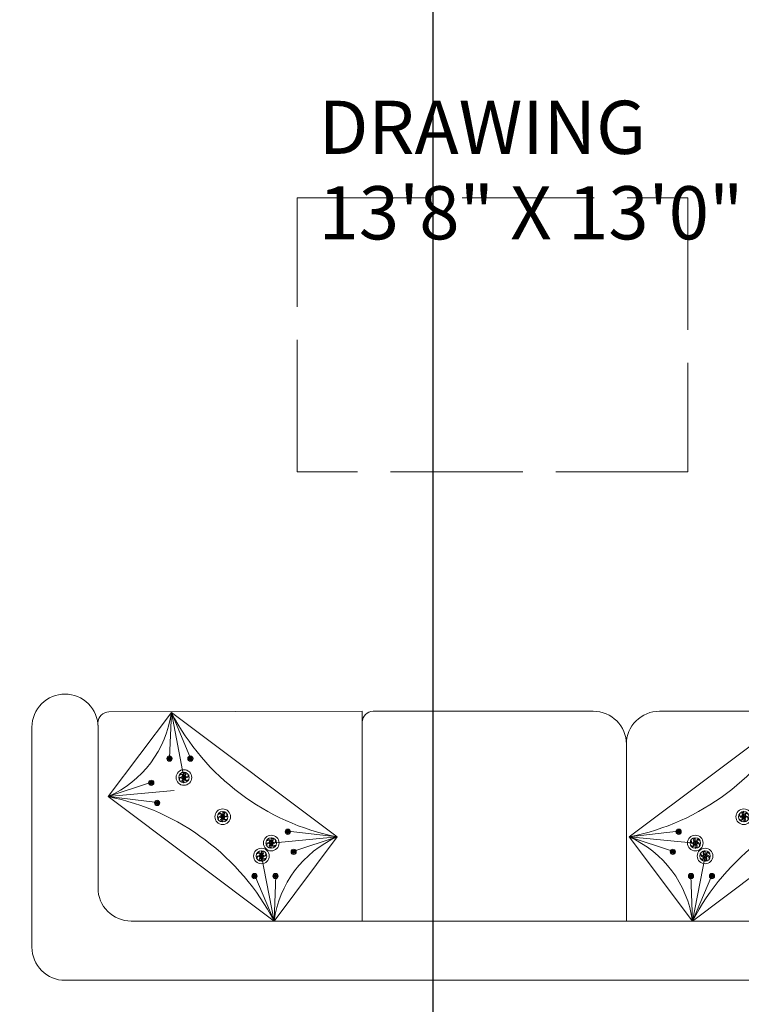
# Model space of a CAD drawing. Units: inches. Extents: x -61 to 1599, y -1316 to 257.
# Tile 132 of 204: x 418 to 484, y -166 to -77. Entities that reach past the tile are written whole.
import ezdxf

# ---------------------------------------------------------------- set-up
doc = ezdxf.new("R2010")
doc.units = ezdxf.units.IN
doc.header["$MEASUREMENT"] = 0
doc.linetypes.add('ACAD_ISO02W100', pattern=[15, 12, -3])
for name, color, linetype, lineweight in [('A-ANNO-DIMS', 2, 'Continuous', 18), ('A-AREA-IDEN', 1, 'Continuous', 18), ('A-FURN-LOW', 83, 'ACAD_ISO02W100', 18), ('FURNITURE', 83, 'Continuous', 18)]:
    doc.layers.add(name, color=color, linetype=linetype, lineweight=lineweight)
doc.layers.add('FUR', color=83, linetype='Continuous')
doc.styles.get("Standard").update_dxf_attribs({"font": 'arial.ttf'})
doc.dimstyles.get("Standard").update_dxf_attribs({"dimtxt": 0.18, "dimasz": 0.18, "dimexe": 0.18, "dimexo": 0.0625, "dimgap": 0.09, "dimtad": 0, "dimtih": 1, "dimtoh": 1, "dimdec": 0, "dimzin": 0, "dimdsep": 46, "dimlunit": 3, "dimtxsty": 'Standard', "dimcen": 0.09, "dimadec": 0, "dimazin": 0, "dimtfac": 1, "dimtdec": 0, "dimtofl": 0, "dimtmove": 0, "dimatfit": 3, "dimfxl": 1, "dimtolj": 1, "dimtzin": 0, "dimarcsym": 0})

# ---------------------------------------------------------------- blocks, each defined once
blk = doc.blocks.new('*U152')
at = {"layer": 'FUR'}
blk.add_open_spline([(0.005, 0.08), (-0.03, 0.048), (-0.098, -0.015), (0.075, -0.018), (0.024, -0.063), (0.005, -0.08)], degree=3, knots=[0, 0, 0, 0, 0.0954578, 0.1898773, 0.2470677, 0.2470677, 0.2470677, 0.2470677], dxfattribs=at)
blk = doc.blocks.new('*U153')
at = {"layer": 'FUR', "transparency": 16777216}
for p, rotation in [((222.173, -79.977), 60), ((222.178, -80.056), 120), ((222.25, -80.092), 180), ((222.312, -79.968), 300), ((222.317, -80.048), 240)]:
    blk.add_blockref('*U152', p, dxfattribs=dict(at, rotation=rotation))
blk.add_blockref('*U152', (222.24, -79.932), dxfattribs=at)
blk = doc.blocks.new('*U154')
at = {"layer": 'FUR'}
blk.add_open_spline([(0.005, 0.08), (-0.03, 0.048), (-0.098, -0.015), (0.075, -0.018), (0.024, -0.063), (0.005, -0.08)], degree=3, knots=[0, 0, 0, 0, 0.0954578, 0.1898773, 0.2470677, 0.2470677, 0.2470677, 0.2470677], dxfattribs=at)
blk = doc.blocks.new('*U155')
at = {"layer": 'FUR', "transparency": 16777216}
for p, rotation in [((222.173, -79.977), 60), ((222.178, -80.056), 120), ((222.25, -80.092), 180), ((222.312, -79.968), 300), ((222.317, -80.048), 240)]:
    blk.add_blockref('*U154', p, dxfattribs=dict(at, rotation=rotation))
blk.add_blockref('*U154', (222.24, -79.932), dxfattribs=at)
blk = doc.blocks.new('*U148')
at = {"layer": 'FUR'}
blk.add_open_spline([(0.005, 0.08), (-0.03, 0.048), (-0.098, -0.015), (0.075, -0.018), (0.024, -0.063), (0.005, -0.08)], degree=3, knots=[0, 0, 0, 0, 0.0954578, 0.1898773, 0.2470677, 0.2470677, 0.2470677, 0.2470677], dxfattribs=at)
blk = doc.blocks.new('*U149')
at = {"layer": 'FUR', "transparency": 16777216}
for p, rotation in [((222.173, -79.977), 60), ((222.178, -80.056), 120), ((222.25, -80.092), 180), ((222.312, -79.968), 300), ((222.317, -80.048), 240)]:
    blk.add_blockref('*U148', p, dxfattribs=dict(at, rotation=rotation))
blk.add_blockref('*U148', (222.24, -79.932), dxfattribs=at)
blk = doc.blocks.new('*U128')
at = {"layer": 'FUR'}
blk.add_open_spline([(0.015, 0.238), (-0.088, 0.143), (-0.292, -0.045), (0.224, -0.053), (0.072, -0.187), (0.015, -0.238)], degree=3, knots=[0, 0, 0, 0, 0.2846533, 0.5662105, 0.736751, 0.736751, 0.736751, 0.736751], dxfattribs=at)
blk = doc.blocks.new('*U129')
at = {"layer": 'FUR', "transparency": 16777216}
for p, rotation in [((662.517, -238.489), 60), ((662.531, -238.727), 120), ((662.745, -238.833), 180), ((662.929, -238.463), 300), ((662.944, -238.702), 240)]:
    blk.add_blockref('*U128', p, dxfattribs=dict(at, rotation=rotation))
blk.add_blockref('*U128', (662.716, -238.357), dxfattribs=at)
blk = doc.blocks.new('*U150')
at = {"layer": 'FUR'}
blk.add_open_spline([(0.005, 0.08), (-0.03, 0.048), (-0.098, -0.015), (0.075, -0.018), (0.024, -0.063), (0.005, -0.08)], degree=3, knots=[0, 0, 0, 0, 0.0954578, 0.1898773, 0.2470677, 0.2470677, 0.2470677, 0.2470677], dxfattribs=at)
blk = doc.blocks.new('*U151')
at = {"layer": 'FUR', "transparency": 16777216}
for p, rotation in [((222.173, -79.977), 60), ((222.178, -80.056), 120), ((222.25, -80.092), 180), ((222.312, -79.968), 300), ((222.317, -80.048), 240)]:
    blk.add_blockref('*U150', p, dxfattribs=dict(at, rotation=rotation))
blk.add_blockref('*U150', (222.24, -79.932), dxfattribs=at)
blk = doc.blocks.new('*U132')
at = {"layer": 'FUR'}
blk.add_open_spline([(0.015, 0.238), (-0.088, 0.143), (-0.292, -0.045), (0.224, -0.053), (0.072, -0.187), (0.015, -0.238)], degree=3, knots=[0, 0, 0, 0, 0.2846533, 0.5662105, 0.736751, 0.736751, 0.736751, 0.736751], dxfattribs=at)
blk = doc.blocks.new('*U133')
at = {"layer": 'FUR', "transparency": 16777216}
for p, rotation in [((662.517, -238.489), 60), ((662.531, -238.727), 120), ((662.745, -238.833), 180), ((662.929, -238.463), 300), ((662.944, -238.702), 240)]:
    blk.add_blockref('*U132', p, dxfattribs=dict(at, rotation=rotation))
blk.add_blockref('*U132', (662.716, -238.357), dxfattribs=at)
blk = doc.blocks.new('*U124')
at = {"layer": 'FUR'}
blk.add_open_spline([(0.005, 0.08), (-0.03, 0.048), (-0.098, -0.015), (0.075, -0.018), (0.024, -0.063), (0.005, -0.08)], degree=3, knots=[0, 0, 0, 0, 0.0954578, 0.1898773, 0.2470677, 0.2470677, 0.2470677, 0.2470677], dxfattribs=at)
blk = doc.blocks.new('*U125')
at = {"layer": 'FUR', "transparency": 16777216}
for p, rotation in [((222.173, -79.977), 60), ((222.178, -80.056), 120), ((222.25, -80.092), 180), ((222.312, -79.968), 300), ((222.317, -80.048), 240)]:
    blk.add_blockref('*U124', p, dxfattribs=dict(at, rotation=rotation))
blk.add_blockref('*U124', (222.24, -79.932), dxfattribs=at)
blk = doc.blocks.new('*U134')
at = {"layer": 'FUR'}
blk.add_open_spline([(0.015, 0.238), (-0.088, 0.143), (-0.292, -0.045), (0.224, -0.053), (0.072, -0.187), (0.015, -0.238)], degree=3, knots=[0, 0, 0, 0, 0.2846533, 0.5662105, 0.736751, 0.736751, 0.736751, 0.736751], dxfattribs=at)
blk = doc.blocks.new('*U123')
at = {"layer": 'FUR', "transparency": 16777216}
for p, rotation in [((662.517, -238.489), 60), ((662.531, -238.727), 120), ((662.745, -238.833), 180), ((662.929, -238.463), 300), ((662.944, -238.702), 240)]:
    blk.add_blockref('*U134', p, dxfattribs=dict(at, rotation=rotation))
blk.add_blockref('*U134', (662.716, -238.357), dxfattribs=at)
blk = doc.blocks.new('*U130')
at = {"layer": 'FUR'}
blk.add_open_spline([(0.015, 0.238), (-0.088, 0.143), (-0.292, -0.045), (0.224, -0.053), (0.072, -0.187), (0.015, -0.238)], degree=3, knots=[0, 0, 0, 0, 0.2846533, 0.5662105, 0.736751, 0.736751, 0.736751, 0.736751], dxfattribs=at)
blk = doc.blocks.new('*U131')
at = {"layer": 'FUR', "transparency": 16777216}
for p, rotation in [((662.517, -238.489), 60), ((662.531, -238.727), 120), ((662.745, -238.833), 180), ((662.929, -238.463), 300), ((662.944, -238.702), 240)]:
    blk.add_blockref('*U130', p, dxfattribs=dict(at, rotation=rotation))
blk.add_blockref('*U130', (662.716, -238.357), dxfattribs=at)
blk = doc.blocks.new('*U126')
at = {"layer": 'FUR'}
blk.add_open_spline([(0.005, 0.08), (-0.03, 0.048), (-0.098, -0.015), (0.075, -0.018), (0.024, -0.063), (0.005, -0.08)], degree=3, knots=[0, 0, 0, 0, 0.0954578, 0.1898773, 0.2470677, 0.2470677, 0.2470677, 0.2470677], dxfattribs=at)
blk = doc.blocks.new('*U127')
at = {"layer": 'FUR', "transparency": 16777216}
for p, rotation in [((222.173, -79.977), 60), ((222.178, -80.056), 120), ((222.25, -80.092), 180), ((222.312, -79.968), 300), ((222.317, -80.048), 240)]:
    blk.add_blockref('*U126', p, dxfattribs=dict(at, rotation=rotation))
blk.add_blockref('*U126', (222.24, -79.932), dxfattribs=at)
blk = doc.blocks.new('*U146')
at = {"layer": 'FUR'}
blk.add_open_spline([(0.005, 0.08), (-0.03, 0.048), (-0.098, -0.015), (0.075, -0.018), (0.024, -0.063), (0.005, -0.08)], degree=3, knots=[0, 0, 0, 0, 0.0954578, 0.1898773, 0.2470677, 0.2470677, 0.2470677, 0.2470677], dxfattribs=at)
blk = doc.blocks.new('*U147')
at = {"layer": 'FUR', "transparency": 16777216}
for p, rotation in [((222.173, -79.977), 60), ((222.178, -80.056), 120), ((222.25, -80.092), 180), ((222.312, -79.968), 300), ((222.317, -80.048), 240)]:
    blk.add_blockref('*U146', p, dxfattribs=dict(at, rotation=rotation))
blk.add_blockref('*U146', (222.24, -79.932), dxfattribs=at)
blk = doc.blocks.new('*U144')
at = {"layer": 'FUR'}
blk.add_open_spline([(0.005, 0.08), (-0.03, 0.048), (-0.098, -0.015), (0.075, -0.018), (0.024, -0.063), (0.005, -0.08)], degree=3, knots=[0, 0, 0, 0, 0.0954578, 0.1898773, 0.2470677, 0.2470677, 0.2470677, 0.2470677], dxfattribs=at)
blk = doc.blocks.new('*U145')
at = {"layer": 'FUR', "transparency": 16777216}
for p, rotation in [((222.173, -79.977), 60), ((222.178, -80.056), 120), ((222.25, -80.092), 180), ((222.312, -79.968), 300), ((222.317, -80.048), 240)]:
    blk.add_blockref('*U144', p, dxfattribs=dict(at, rotation=rotation))
blk.add_blockref('*U144', (222.24, -79.932), dxfattribs=at)
blk = doc.blocks.new('*U114')
at = {"layer": 'FUR'}
blk.add_open_spline([(0.005, 0.08), (-0.03, 0.048), (-0.098, -0.015), (0.075, -0.018), (0.024, -0.063), (0.005, -0.08)], degree=3, knots=[0, 0, 0, 0, 0.0954578, 0.1898773, 0.2470677, 0.2470677, 0.2470677, 0.2470677], dxfattribs=at)
blk = doc.blocks.new('*U115')
at = {"layer": 'FUR', "transparency": 16777216}
for p, rotation in [((222.173, -79.977), 60), ((222.178, -80.056), 120), ((222.25, -80.092), 180), ((222.312, -79.968), 300), ((222.317, -80.048), 240)]:
    blk.add_blockref('*U114', p, dxfattribs=dict(at, rotation=rotation))
blk.add_blockref('*U114', (222.24, -79.932), dxfattribs=at)
blk = doc.blocks.new('*U116')
at = {"layer": 'FUR'}
blk.add_open_spline([(0.005, 0.08), (-0.03, 0.048), (-0.098, -0.015), (0.075, -0.018), (0.024, -0.063), (0.005, -0.08)], degree=3, knots=[0, 0, 0, 0, 0.0954578, 0.1898773, 0.2470677, 0.2470677, 0.2470677, 0.2470677], dxfattribs=at)
blk = doc.blocks.new('*U117')
at = {"layer": 'FUR', "transparency": 16777216}
for p, rotation in [((222.173, -79.977), 60), ((222.178, -80.056), 120), ((222.25, -80.092), 180), ((222.312, -79.968), 300), ((222.317, -80.048), 240)]:
    blk.add_blockref('*U116', p, dxfattribs=dict(at, rotation=rotation))
blk.add_blockref('*U116', (222.24, -79.932), dxfattribs=at)
blk = doc.blocks.new('*U112')
at = {"layer": 'FUR'}
blk.add_open_spline([(0.005, 0.08), (-0.03, 0.048), (-0.098, -0.015), (0.075, -0.018), (0.024, -0.063), (0.005, -0.08)], degree=3, knots=[0, 0, 0, 0, 0.0954578, 0.1898773, 0.2470677, 0.2470677, 0.2470677, 0.2470677], dxfattribs=at)
blk = doc.blocks.new('*U113')
at = {"layer": 'FUR', "transparency": 16777216}
for p, rotation in [((222.173, -79.977), 60), ((222.178, -80.056), 120), ((222.25, -80.092), 180), ((222.312, -79.968), 300), ((222.317, -80.048), 240)]:
    blk.add_blockref('*U112', p, dxfattribs=dict(at, rotation=rotation))
blk.add_blockref('*U112', (222.24, -79.932), dxfattribs=at)
blk = doc.blocks.new('*U142')
at = {"layer": 'FUR'}
blk.add_open_spline([(0.015, 0.238), (-0.088, 0.143), (-0.292, -0.045), (0.224, -0.053), (0.072, -0.187), (0.015, -0.238)], degree=3, knots=[0, 0, 0, 0, 0.2846533, 0.5662105, 0.736751, 0.736751, 0.736751, 0.736751], dxfattribs=at)
blk = doc.blocks.new('*U143')
at = {"layer": 'FUR', "transparency": 16777216}
for p, rotation in [((662.517, -238.489), 60), ((662.531, -238.727), 120), ((662.745, -238.833), 180), ((662.929, -238.463), 300), ((662.944, -238.702), 240)]:
    blk.add_blockref('*U142', p, dxfattribs=dict(at, rotation=rotation))
blk.add_blockref('*U142', (662.716, -238.357), dxfattribs=at)
blk = doc.blocks.new('*U158')
at = {"layer": 'FUR'}
blk.add_open_spline([(0.015, 0.238), (-0.088, 0.143), (-0.292, -0.045), (0.224, -0.053), (0.072, -0.187), (0.015, -0.238)], degree=3, knots=[0, 0, 0, 0, 0.2846533, 0.5662105, 0.736751, 0.736751, 0.736751, 0.736751], dxfattribs=at)
blk = doc.blocks.new('*U109')
at = {"layer": 'FUR', "transparency": 16777216}
for p, rotation in [((662.517, -238.489), 60), ((662.531, -238.727), 120), ((662.745, -238.833), 180), ((662.929, -238.463), 300), ((662.944, -238.702), 240)]:
    blk.add_blockref('*U158', p, dxfattribs=dict(at, rotation=rotation))
blk.add_blockref('*U158', (662.716, -238.357), dxfattribs=at)
blk = doc.blocks.new('*U110')
at = {"layer": 'FUR'}
blk.add_open_spline([(0.005, 0.08), (-0.03, 0.048), (-0.098, -0.015), (0.075, -0.018), (0.024, -0.063), (0.005, -0.08)], degree=3, knots=[0, 0, 0, 0, 0.0954578, 0.1898773, 0.2470677, 0.2470677, 0.2470677, 0.2470677], dxfattribs=at)
blk = doc.blocks.new('*U111')
at = {"layer": 'FUR', "transparency": 16777216}
for p, rotation in [((222.173, -79.977), 60), ((222.178, -80.056), 120), ((222.25, -80.092), 180), ((222.312, -79.968), 300), ((222.317, -80.048), 240)]:
    blk.add_blockref('*U110', p, dxfattribs=dict(at, rotation=rotation))
blk.add_blockref('*U110', (222.24, -79.932), dxfattribs=at)
blk = doc.blocks.new('*U156')
at = {"layer": 'FUR'}
blk.add_open_spline([(0.015, 0.238), (-0.088, 0.143), (-0.292, -0.045), (0.224, -0.053), (0.072, -0.187), (0.015, -0.238)], degree=3, knots=[0, 0, 0, 0, 0.2846533, 0.5662105, 0.736751, 0.736751, 0.736751, 0.736751], dxfattribs=at)
blk = doc.blocks.new('*U157')
at = {"layer": 'FUR', "transparency": 16777216}
for p, rotation in [((662.517, -238.489), 60), ((662.531, -238.727), 120), ((662.745, -238.833), 180), ((662.929, -238.463), 300), ((662.944, -238.702), 240)]:
    blk.add_blockref('*U156', p, dxfattribs=dict(at, rotation=rotation))
blk.add_blockref('*U156', (662.716, -238.357), dxfattribs=at)
blk = doc.blocks.new('*U120')
at = {"layer": 'FUR'}
blk.add_open_spline([(0.005, 0.08), (-0.03, 0.048), (-0.098, -0.015), (0.075, -0.018), (0.024, -0.063), (0.005, -0.08)], degree=3, knots=[0, 0, 0, 0, 0.0954578, 0.1898773, 0.2470677, 0.2470677, 0.2470677, 0.2470677], dxfattribs=at)
blk = doc.blocks.new('*U121')
at = {"layer": 'FUR', "transparency": 16777216}
for p, rotation in [((222.173, -79.977), 60), ((222.178, -80.056), 120), ((222.25, -80.092), 180), ((222.312, -79.968), 300), ((222.317, -80.048), 240)]:
    blk.add_blockref('*U120', p, dxfattribs=dict(at, rotation=rotation))
blk.add_blockref('*U120', (222.24, -79.932), dxfattribs=at)
blk = doc.blocks.new('*U140')
at = {"layer": 'FUR'}
blk.add_open_spline([(0.015, 0.238), (-0.088, 0.143), (-0.292, -0.045), (0.224, -0.053), (0.072, -0.187), (0.015, -0.238)], degree=3, knots=[0, 0, 0, 0, 0.2846533, 0.5662105, 0.736751, 0.736751, 0.736751, 0.736751], dxfattribs=at)
blk = doc.blocks.new('*U141')
at = {"layer": 'FUR', "transparency": 16777216}
for p, rotation in [((662.517, -238.489), 60), ((662.531, -238.727), 120), ((662.745, -238.833), 180), ((662.929, -238.463), 300), ((662.944, -238.702), 240)]:
    blk.add_blockref('*U140', p, dxfattribs=dict(at, rotation=rotation))
blk.add_blockref('*U140', (662.716, -238.357), dxfattribs=at)
blk = doc.blocks.new('*U135')
at = {"layer": 'FUR'}
blk.add_open_spline([(0.015, 0.238), (-0.088, 0.143), (-0.292, -0.045), (0.224, -0.053), (0.072, -0.187), (0.015, -0.238)], degree=3, knots=[0, 0, 0, 0, 0.2846533, 0.5662105, 0.736751, 0.736751, 0.736751, 0.736751], dxfattribs=at)
blk = doc.blocks.new('*U136')
at = {"layer": 'FUR', "transparency": 16777216}
for p, rotation in [((662.517, -238.489), 60), ((662.531, -238.727), 120), ((662.745, -238.833), 180), ((662.929, -238.463), 300), ((662.944, -238.702), 240)]:
    blk.add_blockref('*U135', p, dxfattribs=dict(at, rotation=rotation))
blk.add_blockref('*U135', (662.716, -238.357), dxfattribs=at)
blk = doc.blocks.new('*U118')
at = {"layer": 'FUR'}
blk.add_open_spline([(0.005, 0.08), (-0.03, 0.048), (-0.098, -0.015), (0.075, -0.018), (0.024, -0.063), (0.005, -0.08)], degree=3, knots=[0, 0, 0, 0, 0.0954578, 0.1898773, 0.2470677, 0.2470677, 0.2470677, 0.2470677], dxfattribs=at)
blk = doc.blocks.new('*U119')
at = {"layer": 'FUR', "transparency": 16777216}
for p, rotation in [((222.173, -79.977), 60), ((222.178, -80.056), 120), ((222.25, -80.092), 180), ((222.312, -79.968), 300), ((222.317, -80.048), 240)]:
    blk.add_blockref('*U118', p, dxfattribs=dict(at, rotation=rotation))
blk.add_blockref('*U118', (222.24, -79.932), dxfattribs=at)
blk = doc.blocks.new('*U138')
at = {"layer": 'FUR'}
blk.add_open_spline([(0.005, 0.08), (-0.03, 0.048), (-0.098, -0.015), (0.075, -0.018), (0.024, -0.063), (0.005, -0.08)], degree=3, knots=[0, 0, 0, 0, 0.0954578, 0.1898773, 0.2470677, 0.2470677, 0.2470677, 0.2470677], dxfattribs=at)
blk = doc.blocks.new('*U139')
at = {"layer": 'FUR', "transparency": 16777216}
for p, rotation in [((222.173, -79.977), 60), ((222.178, -80.056), 120), ((222.25, -80.092), 180), ((222.312, -79.968), 300), ((222.317, -80.048), 240)]:
    blk.add_blockref('*U138', p, dxfattribs=dict(at, rotation=rotation))
blk.add_blockref('*U138', (222.24, -79.932), dxfattribs=at)
blk = doc.blocks.new('*U122')
at = {"layer": 'FUR'}
blk.add_open_spline([(0.005, 0.08), (-0.03, 0.048), (-0.098, -0.015), (0.075, -0.018), (0.024, -0.063), (0.005, -0.08)], degree=3, knots=[0, 0, 0, 0, 0.0954578, 0.1898773, 0.2470677, 0.2470677, 0.2470677, 0.2470677], dxfattribs=at)
blk = doc.blocks.new('*U137')
at = {"layer": 'FUR', "transparency": 16777216}
for p, rotation in [((222.173, -79.977), 60), ((222.178, -80.056), 120), ((222.25, -80.092), 180), ((222.312, -79.968), 300), ((222.317, -80.048), 240)]:
    blk.add_blockref('*U122', p, dxfattribs=dict(at, rotation=rotation))
blk.add_blockref('*U122', (222.24, -79.932), dxfattribs=at)
blk = doc.blocks.new('SOFA-THREE-SEAT')
for p, q in [((30, 24.442), (6.996, 24.38)), ((12.664, 24.333), (12.509, 20.192)), ((12.664, 24.333), (13.805, 18.423)), ((12.664, 24.333), (14.414, 20.192)), ((30, 23.442), (29.997, 24.442)), ((51, 24.442), (31, 24.442)), ((78.369, 24.442), (57, 24.442)), ((69.336, 24.333), (67.586, 20.192)), ((69.336, 24.333), (68.194, 18.423)), ((69.336, 24.333), (69.49, 20.192)), ((6, 23), (5.999, 23.377)), ((30, 23.442), (30, 5.382)), ((54, 21.442), (54, 5.382)), ((54, 21.442), (54, 21.442)), ((12.49, 20.139), (12.49, 20.299)), ((12.49, 20.139), (12.49, 19.979)), ((14.394, 20.139), (14.394, 20.299)), ((14.394, 20.139), (14.394, 19.979)), ((67.605, 20.139), (67.605, 20.299)), ((67.605, 20.139), (67.605, 19.979)), ((69.509, 20.139), (69.509, 20.299)), ((69.509, 20.139), (69.509, 19.979)), ((13.805, 18.423), (13.805, 18.899)), ((68.194, 18.423), (68.194, 18.899)), ((6.926, 16.687), (10.859, 17.993)), ((10.84, 17.94), (10.84, 18.1)), ((10.84, 17.94), (10.84, 17.78)), ((13.805, 18.423), (13.805, 17.946)), ((68.194, 18.423), (68.194, 17.946)), ((75.074, 16.687), (71.14, 17.993)), ((71.159, 17.94), (71.159, 18.1)), ((71.159, 17.94), (71.159, 17.78)), ((6.926, 16.687), (12.92, 17.243)), ((69.079, 17.243), (69.079, 17.719)), ((75.074, 16.687), (69.079, 17.243)), ((69.079, 17.243), (69.079, 16.766)), ((6.926, 16.687), (11.391, 16.164)), ((11.372, 16.112), (11.372, 16.272)), ((11.372, 16.112), (11.372, 15.952)), ((75.074, 16.687), (70.608, 16.164)), ((70.627, 16.112), (70.627, 16.272)), ((70.627, 16.112), (70.627, 15.952)), ((17.327, 14.857), (17.327, 15.334)), ((64.672, 14.857), (64.672, 15.334)), ((17.327, 14.857), (17.327, 14.381)), ((64.672, 14.857), (64.672, 14.381)), ((23.243, 13.498), (23.243, 13.658)), ((23.243, 13.498), (23.243, 13.338)), ((27.729, 13.028), (23.263, 13.551)), ((54.271, 13.028), (58.736, 13.551)), ((58.756, 13.498), (58.756, 13.658)), ((58.756, 13.498), (58.756, 13.338)), ((27.729, 13.028), (21.735, 12.472)), ((21.735, 12.472), (21.735, 12.949)), ((27.729, 13.028), (23.795, 11.722)), ((54.271, 13.028), (60.265, 12.472)), ((54.271, 13.028), (58.204, 11.722)), ((60.265, 12.472), (60.265, 12.949)), ((20.849, 11.292), (20.849, 11.769)), ((21.735, 12.472), (21.735, 11.996)), ((23.776, 11.67), (23.776, 11.83)), ((23.776, 11.67), (23.776, 11.51)), ((58.224, 11.67), (58.224, 11.83)), ((58.224, 11.67), (58.224, 11.51)), ((60.265, 12.472), (60.265, 11.996)), ((61.15, 11.292), (61.15, 11.769)), ((21.991, 5.382), (20.849, 11.292)), ((20.849, 11.292), (20.849, 10.816)), ((60.009, 5.382), (61.15, 11.292)), ((61.15, 11.292), (61.15, 10.816)), ((20.221, 9.471), (20.221, 9.631)), ((20.221, 9.471), (20.221, 9.311)), ((21.991, 5.382), (20.241, 9.523)), ((21.991, 5.382), (22.145, 9.523)), ((22.125, 9.471), (22.125, 9.631)), ((22.125, 9.471), (22.125, 9.311)), ((60.009, 5.382), (59.854, 9.523)), ((59.874, 9.471), (59.874, 9.631)), ((59.874, 9.471), (59.874, 9.311)), ((60.009, 5.382), (61.759, 9.523)), ((61.778, 9.471), (61.778, 9.631)), ((61.778, 9.471), (61.778, 9.311))]:
    blk.add_line(p, q)
blk.add_lwpolyline([(78, 8.382), (78, 23, -0.414214), (81, 26), (81, 26, -0.414214), (84, 23), (84, 3, -0.414214), (81, 0), (3, 0, -0.414214), (0, 3), (0, 23, -0.414214), (3, 26), (3, 26, -0.414214), (6, 23), (6, 8.382, 0.414214), (9, 5.382), (75, 5.382, 0.414214)], format="xyb", close=True)
for points in [[(27.729, 13.028), (12.664, 24.333), (6.926, 16.687), (21.991, 5.382)], [(54.271, 13.028), (69.336, 24.333), (75.074, 16.687), (60.009, 5.382)]]:
    blk.add_lwpolyline(points, close=True)
for centre, radius in [((12.49, 20.139), 0.238), ((12.49, 20.139), 0.16), ((14.394, 20.139), 0.238), ((14.394, 20.139), 0.16), ((67.605, 20.139), 0.238), ((67.605, 20.139), 0.16), ((69.509, 20.139), 0.238), ((69.509, 20.139), 0.16), ((13.805, 18.423), 0.71), ((13.805, 18.423), 0.476), ((68.194, 18.423), 0.71), ((68.194, 18.423), 0.476), ((10.84, 17.94), 0.238), ((10.84, 17.94), 0.16), ((69.079, 17.243), 0.71), ((71.159, 17.94), 0.238), ((71.159, 17.94), 0.16), ((69.079, 17.243), 0.476), ((11.372, 16.112), 0.238), ((11.372, 16.112), 0.16), ((70.627, 16.112), 0.238), ((70.627, 16.112), 0.16), ((17.327, 14.857), 0.71), ((17.327, 14.857), 0.476), ((64.672, 14.857), 0.71), ((64.672, 14.857), 0.476), ((23.243, 13.498), 0.238), ((23.243, 13.498), 0.16), ((58.756, 13.498), 0.238), ((58.756, 13.498), 0.16), ((21.735, 12.472), 0.71), ((21.735, 12.472), 0.476), ((60.265, 12.472), 0.71), ((60.265, 12.472), 0.476), ((20.849, 11.292), 0.71), ((20.849, 11.292), 0.476), ((23.776, 11.67), 0.238), ((23.776, 11.67), 0.16), ((58.224, 11.67), 0.238), ((58.224, 11.67), 0.16), ((61.15, 11.292), 0.71), ((61.15, 11.292), 0.476), ((20.221, 9.471), 0.238), ((20.221, 9.471), 0.16), ((22.125, 9.471), 0.238), ((22.125, 9.471), 0.16), ((59.874, 9.471), 0.238), ((59.874, 9.471), 0.16), ((61.778, 9.471), 0.238), ((61.778, 9.471), 0.16)]:
    blk.add_circle(centre, radius)
for centre, radius, start, end in [((6.999, 23.38), 1, 90.15417, 180.15417), ((2.937, 25.656), 9.816, 293.97422, 352.25297), ((31.951, 34.345), 21.731, 207.43163, 258.79556), ((31, 23.442), 1, 89.99998, 179.99998), ((51, 21.442), 3, 359.99998, 89.99998), ((57, 21.442), 3, 90, 180.00002), ((50.048, 34.345), 21.731, 281.20444, 332.56837), ((79.062, 25.656), 9.816, 187.74703, 246.02578), ((2.703, -4.63), 21.731, 27.43163, 78.79556), ((79.296, -4.63), 21.731, 101.20444, 152.56837), ((31.717, 4.059), 9.816, 113.97422, 172.25297), ((50.282, 4.059), 9.816, 7.74703, 66.02578)]:
    blk.add_arc(centre, radius, start, end)
at = {"xscale": -1, "rotation": 180}
for name, p in [('*U149', (-209.755, -59.873)), ('*U151', (-207.851, -59.873)), ('*U129', (-648.925, -220.172)), ('*U153', (-211.405, -62.072)), ('*U155', (-210.873, -63.9)), ('*U133', (-645.403, -223.738)), ('*U147', (-199.001, -66.514)), ('*U131', (-640.996, -226.123)), ('*U123', (-641.881, -227.303)), ('*U145', (-198.469, -68.342)), ('*U125', (-202.024, -70.541)), ('*U127', (-200.12, -70.541))]:
    blk.add_blockref(name, p, dxfattribs=at)
at = {"rotation": 180}
for name, p in [('*U121', (289.85, -59.873)), ('*U119', (291.754, -59.873)), ('*U141', (730.924, -220.172)), ('*U137', (293.404, -62.072)), ('*U136', (731.81, -221.352)), ('*U139', (292.872, -63.9)), ('*U157', (727.402, -223.738)), ('*U117', (281.001, -66.514)), ('*U143', (722.995, -226.123)), ('*U115', (280.469, -68.342)), ('*U109', (723.88, -227.303)), ('*U113', (282.119, -70.541)), ('*U111', (284.023, -70.541))]:
    blk.add_blockref(name, p, dxfattribs=at)
blk = doc.blocks.new('*D703')
at = {"layer": 'A-ANNO-DIMS', "color": 0, "lineweight": -2, "transparency": 16777216}
for p, q in [((372.32, -616.882), (372.32, 257.457)), ((372.5, 257.277), (413.7, 257.277)), ((455.653, 257.277), (414.453, 257.277)), ((455.833, -616.882), (455.833, 257.457))]:
    blk.add_line(p, q, dxfattribs=at)
at = {"layer": 'A-ANNO-DIMS', "color": 0, "transparency": 16777216}
for points in [[(372.5, 257.307), (372.5, 257.247), (372.32, 257.277)], [(455.653, 257.307), (455.653, 257.247), (455.833, 257.277)]]:
    blk.add_solid(points, dxfattribs=at)
at = {"layer": 'DEFPOINTS', "color": 0, "transparency": 16777216}
for p in [(455.833, 257.277), (372.32, -616.945), (455.833, -616.945)]:
    blk.add_point(p, dxfattribs=at)
at = {"layer": 'A-ANNO-DIMS', "color": 0, "transparency": 16777216, "insert": (414.076, 257.277), "char_height": 0.18, "attachment_point": 5}
blk.add_mtext('\\A1;83.51', dxfattribs=at)

msp = doc.modelspace()

# ---------------------------------------------------------------- linework, layer by layer
at = {"layer": 'A-FURN-LOW'}
msp.add_lwpolyline([(478.9662, -117.9559), (443.4644, -117.9559), (443.4644, -93.0522), (478.9662, -93.0522)], close=True, dxfattribs=at)

# ---------------------------------------------------------------- block references
at = {"layer": 'FURNITURE'}
msp.add_blockref('SOFA-THREE-SEAT', (419.3851, -164.1303), dxfattribs=at)

# ---------------------------------------------------------------- texts
at = {"layer": 'A-AREA-IDEN'}
for s, height, p in [('DRAWING', 4.8321, (445.4206, -89.0692)), ('13\'8" X 13\'0"', 4.832098, (445.4206, -96.8315))]:
    msp.add_text(s, height=height, dxfattribs=at).set_placement(p)

# ---------------------------------------------------------------- dimensions: what is measured, and where the dimension line sits
at = {"layer": 'A-ANNO-DIMS'}
dim = msp.add_linear_dim(base=(455.8327, 257.2771), p1=(372.3201, -616.9446), p2=(455.8327, -616.9446), dimstyle='Standard', override={"dimdec": 2, "dimlfac": 1, "dimrnd": 0, "dimzin": 0, "dimdsep": 46, "dimlunit": 2}, dxfattribs=at)
dim.commit()
dim.dimension.update_dxf_attribs({"geometry": '*D703', "text_midpoint": (414.0764, 257.2771)})

doc.saveas('drawing.dxf')
